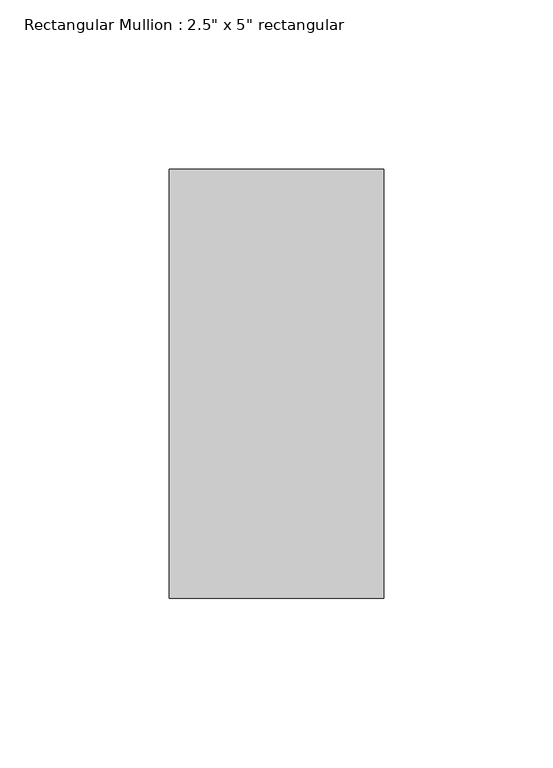
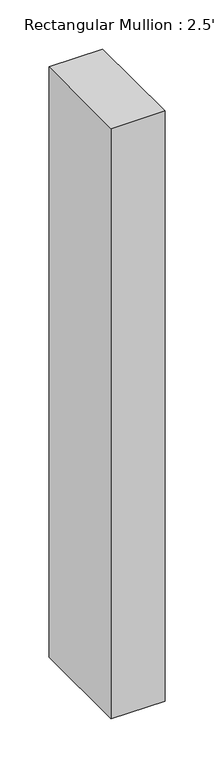
"""IFC4 building model written with IfcOpenShell, lengths in millimetres: member geometry."""

from ifc_helpers import new_model, si_unit, frame, origin, place, context, project, spatial, polyline, outline, extrude, source, transform, mapped, element, save


def member_b91b5e2d(model_context):
    return source(origin(), model_context, "Body", "SweptSolid", [
        extrude(outline(polyline([(0.0, 63.5), (0.0, -63.5), (-63.5, -63.5), (-63.5, 63.5), (0.0, 63.5)])), frame((0.0, 0.0, -734.4018025), z_axis=(0.0, 0.0, 1.0), x_axis=(1.0, 0.0, 0.0)), (0.0, 0.0, 1.0), 734.4018025),
    ])


if __name__ == "__main__":
    model = new_model("IFC4")
    model_context = context("Model", 3, world=origin())
    ifc_project = project(units=[si_unit("LENGTHUNIT", "METRE", prefix="MILLI")], contexts=[model_context])
    site = spatial("IfcSite", under=ifc_project)
    building = spatial("IfcBuilding", under=site)
    placement = place(None, origin())
    member_shape = member_b91b5e2d(model_context)
    element("IfcMember", 1, ObjectType="Rectangular Mullion : 2.5\" x 5\" rectangular", at=placement, inside=building, context=model_context, shape_type="MappedRepresentation", body=[
        mapped(member_shape, transform((0.0, 0.0, 0.0), x_axis=(1.0, 0.0, 0.0), y_axis=(0.0, 1.0, 0.0), z_axis=(0.0, 0.0, 1.0))),
    ])
    save(model, "model.ifc")

# Revit data of these elements
# Type "Rectangular Mullion : 2.5\" x 5\" rectangular"
#   built-in parameter 1007304 = 0.416667 (stored number, unit not read)
#   built-in parameter 1007301 = 0.104167 (stored number, unit not read)
#   built-in parameter 1007300 = 0.104167 (stored number, unit not read)
# Element 1 (IfcMember, "Rectangular Mullion : 2.5\" x 5\" rectangular")
#   Materials on its faces: "Aluminum"
# Materials
#   "Aluminum": class "Metal", colour RGB 247 247 247, transparency 0, Description = "Aluminum 6061", Cost = 0
